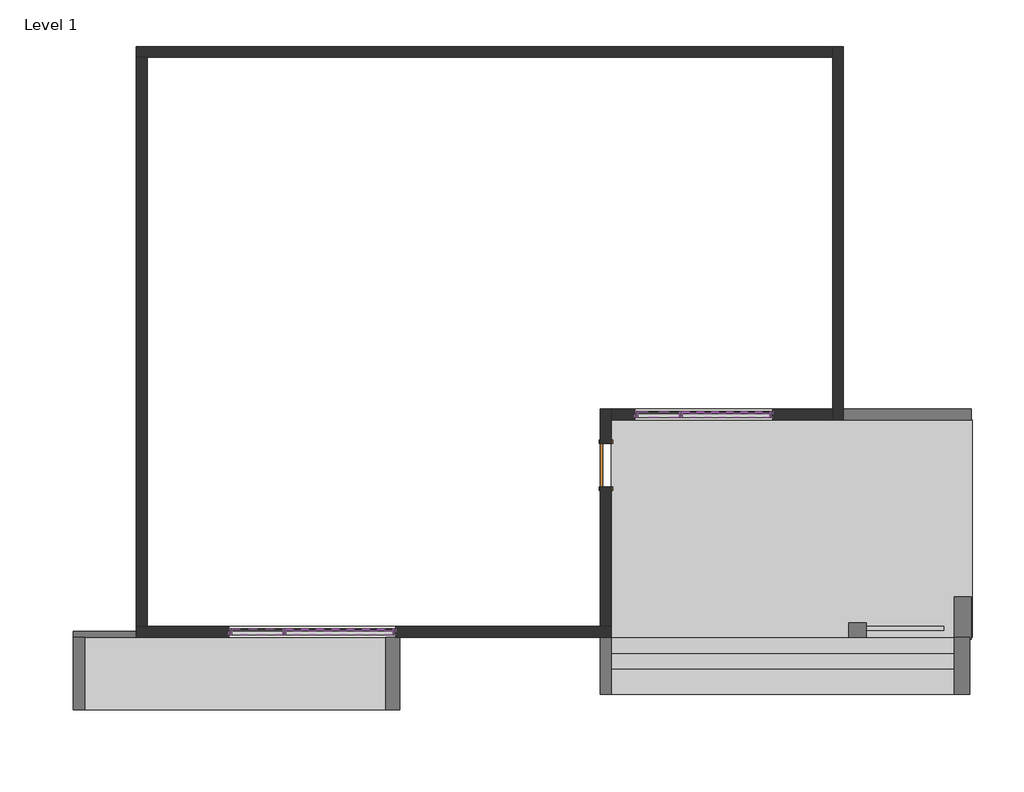
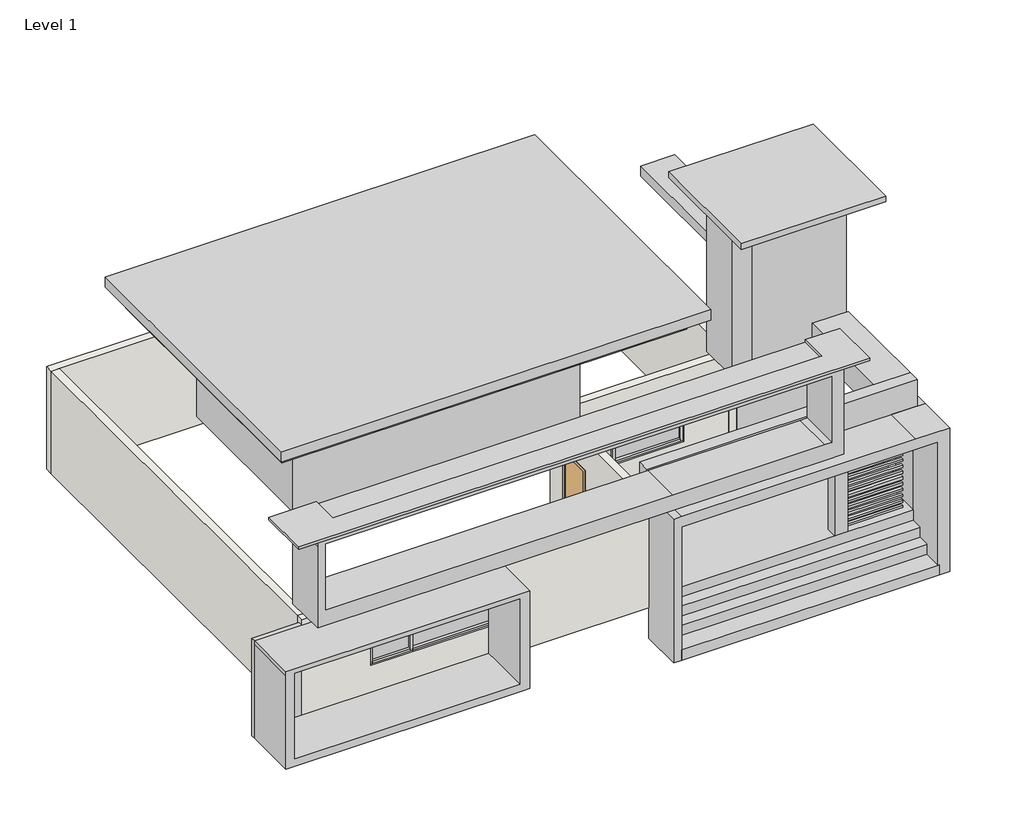
# One storey: 30 members, 8 plates, 6 walls, 5 proxies, 1 door.
"""IFC4 building model written with IfcOpenShell, lengths in millimetres."""

from ifc_helpers import new_model, si_unit, frame, origin, origin_with_axes, place, context, project, spatial, polyline, outline, extrude, faceted_brep, transform, mapped, element, save
from components import generic_models_1_generic_models_1_d0396bf3, generic_models_2_generic_models_2_1e60c849, generic_models_4_generic_models_4_de5db2ce, generic_models_5_generic_models_5_34eadfb7, generic_models_6_generic_models_6_aa42e9c5, door_0ca8825f, member_94e27682, member_024c663a, member_255fa45d, member_75351bdb, member_163b98ee, member_61d667c8, member_4d6ef9b1, member_f3803a17, member_1b8782c9, member_88cd697c, system_panel_glazed_c3c389f2, system_panel_glazed_f495917c, system_panel_glazed_3dd2ea40, system_panel_glazed_ce1b7c8d, system_panel_glazed_f70c9889, system_panel_glazed_55be9c8f

model = new_model("IFC4")

# Units and contexts
model_context = context("Model", 3, world=origin())
ifc_project = project(units=[si_unit("LENGTHUNIT", "METRE", prefix="MILLI")], contexts=[model_context])

# Site, building, storey
site = spatial("IfcSite", under=ifc_project)
building = spatial("IfcBuilding", under=site)
storey = spatial("IfcBuildingStorey", under=building, Name="Level 1", Elevation=0.0)

# Proxies
placement = place(None, origin())
generic_models_1_generic_models_1_shape = generic_models_1_generic_models_1_d0396bf3(model_context)
element("IfcBuildingElementProxy", 1, Name="Generic Models 1 : Generic Models 1", ObjectType="Generic Models 1 : Generic Models 1", at=placement, inside=storey, context=model_context, shape_type="MappedRepresentation", body=[
    mapped(generic_models_1_generic_models_1_shape, transform((0.0, 0.0, 0.0), x_axis=(1.0, 0.0, 0.0), y_axis=(0.0, 1.0, 0.0), z_axis=(0.0, 0.0, 1.0))),
])
generic_models_2_generic_models_2_shape = generic_models_2_generic_models_2_1e60c849(model_context)
element("IfcBuildingElementProxy", 2, Name="Generic Models 2 : Generic Models 2", ObjectType="Generic Models 2 : Generic Models 2", at=placement, inside=storey, context=model_context, shape_type="MappedRepresentation", body=[
    mapped(generic_models_2_generic_models_2_shape, transform((0.0, 0.0, 0.0), x_axis=(1.0, 0.0, 0.0), y_axis=(0.0, 1.0, 0.0), z_axis=(0.0, 0.0, 1.0))),
])
generic_models_4_generic_models_4_shape = generic_models_4_generic_models_4_de5db2ce(model_context)
element("IfcBuildingElementProxy", 3, Name="Generic Models 4 : Generic Models 4", ObjectType="Generic Models 4 : Generic Models 4", at=placement, inside=storey, context=model_context, shape_type="MappedRepresentation", body=[
    mapped(generic_models_4_generic_models_4_shape, transform((0.0, 0.0, 0.0), x_axis=(1.0, 0.0, 0.0), y_axis=(0.0, 1.0, 0.0), z_axis=(0.0, 0.0, 1.0))),
])
generic_models_5_generic_models_5_shape = generic_models_5_generic_models_5_34eadfb7(model_context)
element("IfcBuildingElementProxy", 4, Name="Generic Models 5 : Generic Models 5", ObjectType="Generic Models 5 : Generic Models 5", at=placement, inside=storey, context=model_context, shape_type="MappedRepresentation", body=[
    mapped(generic_models_5_generic_models_5_shape, transform((0.0, 0.0, 0.0), x_axis=(1.0, 0.0, 0.0), y_axis=(0.0, 1.0, 0.0), z_axis=(0.0, 0.0, 1.0))),
])
generic_models_6_generic_models_6_shape = generic_models_6_generic_models_6_aa42e9c5(model_context)
element("IfcBuildingElementProxy", 5, Name="Generic Models 6 : Generic Models 6", ObjectType="Generic Models 6 : Generic Models 6", at=placement, inside=storey, context=model_context, shape_type="MappedRepresentation", body=[
    mapped(generic_models_6_generic_models_6_shape, transform((0.0, 0.0, 0.0), x_axis=(1.0, 0.0, 0.0), y_axis=(0.0, 1.0, 0.0), z_axis=(0.0, 0.0, 1.0))),
])

# Door
door_shape = door_0ca8825f(model_context)
element("IfcDoor", 6, ObjectType="Single-Flush : 36\" x 84\"", at=placement, inside=storey, context=model_context, shape_type="MappedRepresentation", body=[
    mapped(door_shape, transform((-7974.5229687, -7170.2015118, 0.0), x_axis=(0.0, 1.0, 0.0), y_axis=(-1.0, 0.0, 0.0), z_axis=(0.0, 0.0, 1.0))),
])

# Members
member_shape = member_94e27682(model_context)
element("IfcMember", 7, ObjectType="Rectangular Mullion : 2.5\" x 5\" rectangular", at=placement, inside=storey, context=model_context, shape_type="MappedRepresentation", body=[
    mapped(member_shape, transform((-7364.9229687, -6103.4015118, 1983.9447059), x_axis=(-1.0, 0.0, 0.0), y_axis=(0.0, -1.0, 0.0), z_axis=(0.0, 0.0, 1.0))),
])
element("IfcMember", 8, ObjectType="Rectangular Mullion : 2.5\" x 5\" rectangular", at=placement, inside=storey, context=model_context, shape_type="MappedRepresentation", body=[
    mapped(member_shape, transform((-7364.9229687, -6103.4015118, 1439.8060341), x_axis=(-1.0, 0.0, 0.0), y_axis=(0.0, -1.0, 0.0), z_axis=(0.0, 0.0, 1.0))),
])
member_2_shape = member_024c663a(model_context)
element("IfcMember", 9, ObjectType="Rectangular Mullion : 2.5\" x 5\" rectangular", at=placement, inside=storey, context=model_context, shape_type="MappedRepresentation", body=[
    mapped(member_2_shape, transform((-7301.4229687, -6103.4015118, 895.6673623), x_axis=(0.0, 0.0, -1.0), y_axis=(0.0, -1.0, 0.0), z_axis=(-1.0, 0.0, 0.0))),
])
member_3_shape = member_255fa45d(model_context)
element("IfcMember", 10, ObjectType="Rectangular Mullion : 2.5\" x 5\" rectangular", at=placement, inside=storey, context=model_context, shape_type="MappedRepresentation", body=[
    mapped(member_3_shape, transform((-6399.7229687, -6103.4015118, 1439.8060341), x_axis=(1.0, 0.0, 0.0), y_axis=(0.0, -1.0, 0.0), z_axis=(0.0, 0.0, -1.0))),
])
element("IfcMember", 11, ObjectType="Rectangular Mullion : 2.5\" x 5\" rectangular", at=placement, inside=storey, context=model_context, shape_type="MappedRepresentation", body=[
    mapped(member_3_shape, transform((-6399.7229687, -6103.4015118, 895.6673623), x_axis=(1.0, 0.0, 0.0), y_axis=(0.0, -1.0, 0.0), z_axis=(0.0, 0.0, -1.0))),
])
element("IfcMember", 12, ObjectType="Rectangular Mullion : 2.5\" x 5\" rectangular", at=placement, inside=storey, context=model_context, shape_type="MappedRepresentation", body=[
    mapped(member_3_shape, transform((-6399.7229687, -6103.4015118, 1983.9447059), x_axis=(1.0, 0.0, 0.0), y_axis=(0.0, -1.0, 0.0), z_axis=(0.0, 0.0, -1.0))),
])
element("IfcMember", 13, ObjectType="Rectangular Mullion : 2.5\" x 5\" rectangular", at=placement, inside=storey, context=model_context, shape_type="MappedRepresentation", body=[
    mapped(member_2_shape, transform((-6431.4729687, -6103.4015118, 2528.0833777), x_axis=(0.0, 0.0, 1.0), y_axis=(0.0, -1.0, 0.0), z_axis=(1.0, 0.0, 0.0))),
])
element("IfcMember", 14, ObjectType="Rectangular Mullion : 2.5\" x 5\" rectangular", at=placement, inside=storey, context=model_context, shape_type="MappedRepresentation", body=[
    mapped(member_shape, transform((-7364.9229687, -6103.4015118, 2528.0833777), x_axis=(-1.0, 0.0, 0.0), y_axis=(0.0, -1.0, 0.0), z_axis=(0.0, 0.0, 1.0))),
])
member_4_shape = member_75351bdb(model_context)
element("IfcMember", 15, ObjectType="Rectangular Mullion : 2.5\" x 5\" rectangular", at=placement, inside=storey, context=model_context, shape_type="MappedRepresentation", body=[
    mapped(member_4_shape, transform((-6367.9729687, -6103.4015118, 895.6673623), x_axis=(0.0, 0.0, -1.0), y_axis=(0.0, -1.0, 0.0), z_axis=(-1.0, 0.0, 0.0))),
])
member_5_shape = member_163b98ee(model_context)
element("IfcMember", 16, ObjectType="Rectangular Mullion : 2.5\" x 5\" rectangular", at=placement, inside=storey, context=model_context, shape_type="MappedRepresentation", body=[
    mapped(member_5_shape, transform((-4532.8229687, -6103.4015118, 1983.9447059), x_axis=(0.0, 0.0, 1.0), y_axis=(0.0, -1.0, 0.0), z_axis=(1.0, 0.0, 0.0))),
])
element("IfcMember", 17, ObjectType="Rectangular Mullion : 2.5\" x 5\" rectangular", at=placement, inside=storey, context=model_context, shape_type="MappedRepresentation", body=[
    mapped(member_5_shape, transform((-4532.8229687, -6103.4015118, 1439.8060341), x_axis=(0.0, 0.0, 1.0), y_axis=(0.0, -1.0, 0.0), z_axis=(1.0, 0.0, 0.0))),
])
element("IfcMember", 18, ObjectType="Rectangular Mullion : 2.5\" x 5\" rectangular", at=placement, inside=storey, context=model_context, shape_type="MappedRepresentation", body=[
    mapped(member_4_shape, transform((-4532.8229687, -6103.4015118, 2528.0833777), x_axis=(0.0, 0.0, 1.0), y_axis=(0.0, -1.0, 0.0), z_axis=(1.0, 0.0, 0.0))),
])
element("IfcMember", 19, ObjectType="Rectangular Mullion : 2.5\" x 5\" rectangular", at=placement, inside=storey, context=model_context, shape_type="MappedRepresentation", body=[
    mapped(member_shape, transform((-4469.3229687, -6103.4015118, 1439.8060341), x_axis=(1.0, 0.0, 0.0), y_axis=(0.0, -1.0, 0.0), z_axis=(0.0, 0.0, -1.0))),
])
element("IfcMember", 20, ObjectType="Rectangular Mullion : 2.5\" x 5\" rectangular", at=placement, inside=storey, context=model_context, shape_type="MappedRepresentation", body=[
    mapped(member_shape, transform((-4469.3229687, -6103.4015118, 1983.9447059), x_axis=(1.0, 0.0, 0.0), y_axis=(0.0, -1.0, 0.0), z_axis=(0.0, 0.0, -1.0))),
])
element("IfcMember", 21, ObjectType="Rectangular Mullion : 2.5\" x 5\" rectangular", at=placement, inside=storey, context=model_context, shape_type="MappedRepresentation", body=[
    mapped(member_shape, transform((-4469.3229687, -6103.4015118, 895.6673623), x_axis=(1.0, 0.0, 0.0), y_axis=(0.0, -1.0, 0.0), z_axis=(0.0, 0.0, -1.0))),
])
member_6_shape = member_61d667c8(model_context)
element("IfcMember", 22, ObjectType="Rectangular Mullion : 2.5\" x 5\" rectangular", at=placement, inside=storey, context=model_context, shape_type="MappedRepresentation", body=[
    mapped(member_6_shape, transform((-15899.3229687, -10675.4015118, 2116.0432119), x_axis=(-1.0, 0.0, 0.0), y_axis=(0.0, -1.0, 0.0), z_axis=(0.0, 0.0, 1.0))),
])
element("IfcMember", 23, ObjectType="Rectangular Mullion : 2.5\" x 5\" rectangular", at=placement, inside=storey, context=model_context, shape_type="MappedRepresentation", body=[
    mapped(member_6_shape, transform((-15899.3229687, -10675.4015118, 1567.0065378), x_axis=(-1.0, 0.0, 0.0), y_axis=(0.0, -1.0, 0.0), z_axis=(0.0, 0.0, 1.0))),
])
member_7_shape = member_4d6ef9b1(model_context)
element("IfcMember", 24, ObjectType="Rectangular Mullion : 2.5\" x 5\" rectangular", at=placement, inside=storey, context=model_context, shape_type="MappedRepresentation", body=[
    mapped(member_7_shape, transform((-15835.8229687, -10675.4015118, 1017.9698638), x_axis=(0.0, 0.0, -1.0), y_axis=(0.0, -1.0, 0.0), z_axis=(-1.0, 0.0, 0.0))),
])
member_8_shape = member_f3803a17(model_context)
element("IfcMember", 25, ObjectType="Rectangular Mullion : 2.5\" x 5\" rectangular", at=placement, inside=storey, context=model_context, shape_type="MappedRepresentation", body=[
    mapped(member_8_shape, transform((-14730.9229687, -10675.4015118, 1017.9698638), x_axis=(1.0, 0.0, 0.0), y_axis=(0.0, -1.0, 0.0), z_axis=(0.0, 0.0, -1.0))),
])
element("IfcMember", 26, ObjectType="Rectangular Mullion : 2.5\" x 5\" rectangular", at=placement, inside=storey, context=model_context, shape_type="MappedRepresentation", body=[
    mapped(member_8_shape, transform((-14730.9229687, -10675.4015118, 1567.0065378), x_axis=(1.0, 0.0, 0.0), y_axis=(0.0, -1.0, 0.0), z_axis=(0.0, 0.0, -1.0))),
])
element("IfcMember", 27, ObjectType="Rectangular Mullion : 2.5\" x 5\" rectangular", at=placement, inside=storey, context=model_context, shape_type="MappedRepresentation", body=[
    mapped(member_8_shape, transform((-14730.9229687, -10675.4015118, 2116.0432119), x_axis=(1.0, 0.0, 0.0), y_axis=(0.0, -1.0, 0.0), z_axis=(0.0, 0.0, -1.0))),
])
element("IfcMember", 28, ObjectType="Rectangular Mullion : 2.5\" x 5\" rectangular", at=placement, inside=storey, context=model_context, shape_type="MappedRepresentation", body=[
    mapped(member_7_shape, transform((-14762.6729687, -10675.4015118, 2665.0798859), x_axis=(0.0, 0.0, 1.0), y_axis=(0.0, -1.0, 0.0), z_axis=(1.0, 0.0, 0.0))),
])
element("IfcMember", 29, ObjectType="Rectangular Mullion : 2.5\" x 5\" rectangular", at=placement, inside=storey, context=model_context, shape_type="MappedRepresentation", body=[
    mapped(member_6_shape, transform((-15899.3229687, -10675.4015118, 2665.0798859), x_axis=(-1.0, 0.0, 0.0), y_axis=(0.0, -1.0, 0.0), z_axis=(0.0, 0.0, 1.0))),
])
member_9_shape = member_1b8782c9(model_context)
element("IfcMember", 30, ObjectType="Rectangular Mullion : 2.5\" x 5\" rectangular", at=placement, inside=storey, context=model_context, shape_type="MappedRepresentation", body=[
    mapped(member_9_shape, transform((-14699.1729687, -10675.4015118, 1017.9698638), x_axis=(0.0, 0.0, -1.0), y_axis=(0.0, -1.0, 0.0), z_axis=(-1.0, 0.0, 0.0))),
])
member_10_shape = member_88cd697c(model_context)
element("IfcMember", 31, ObjectType="Rectangular Mullion : 2.5\" x 5\" rectangular", at=placement, inside=storey, context=model_context, shape_type="MappedRepresentation", body=[
    mapped(member_10_shape, transform((-12457.6229687, -10675.4015118, 1567.0065378), x_axis=(0.0, 0.0, 1.0), y_axis=(0.0, -1.0, 0.0), z_axis=(1.0, 0.0, 0.0))),
])
element("IfcMember", 32, ObjectType="Rectangular Mullion : 2.5\" x 5\" rectangular", at=placement, inside=storey, context=model_context, shape_type="MappedRepresentation", body=[
    mapped(member_10_shape, transform((-12457.6229687, -10675.4015118, 2116.0432119), x_axis=(0.0, 0.0, 1.0), y_axis=(0.0, -1.0, 0.0), z_axis=(1.0, 0.0, 0.0))),
])
element("IfcMember", 33, ObjectType="Rectangular Mullion : 2.5\" x 5\" rectangular", at=placement, inside=storey, context=model_context, shape_type="MappedRepresentation", body=[
    mapped(member_9_shape, transform((-12457.6229687, -10675.4015118, 2665.0798859), x_axis=(0.0, 0.0, 1.0), y_axis=(0.0, -1.0, 0.0), z_axis=(1.0, 0.0, 0.0))),
])
element("IfcMember", 34, ObjectType="Rectangular Mullion : 2.5\" x 5\" rectangular", at=placement, inside=storey, context=model_context, shape_type="MappedRepresentation", body=[
    mapped(member_6_shape, transform((-12394.1229687, -10675.4015118, 1567.0065378), x_axis=(1.0, 0.0, 0.0), y_axis=(0.0, -1.0, 0.0), z_axis=(0.0, 0.0, -1.0))),
])
element("IfcMember", 35, ObjectType="Rectangular Mullion : 2.5\" x 5\" rectangular", at=placement, inside=storey, context=model_context, shape_type="MappedRepresentation", body=[
    mapped(member_6_shape, transform((-12394.1229687, -10675.4015118, 2116.0432119), x_axis=(1.0, 0.0, 0.0), y_axis=(0.0, -1.0, 0.0), z_axis=(0.0, 0.0, -1.0))),
])
element("IfcMember", 36, ObjectType="Rectangular Mullion : 2.5\" x 5\" rectangular", at=placement, inside=storey, context=model_context, shape_type="MappedRepresentation", body=[
    mapped(member_6_shape, transform((-12394.1229687, -10675.4015118, 1017.9698638), x_axis=(1.0, 0.0, 0.0), y_axis=(0.0, -1.0, 0.0), z_axis=(0.0, 0.0, -1.0))),
])

# Plates
system_panel_glazed_shape = system_panel_glazed_c3c389f2(model_context)
element("IfcPlate", 37, ObjectType="System Panel : Glazed", at=placement, inside=storey, context=model_context, shape_type="MappedRepresentation", body=[
    mapped(system_panel_glazed_shape, transform((-6866.4479687, -6103.4015118, 959.1673623), x_axis=(1.0, 0.0, 0.0), y_axis=(0.0, 1.0, 0.0), z_axis=(0.0, 0.0, 1.0))),
])
system_panel_glazed_2_shape = system_panel_glazed_f495917c(model_context)
element("IfcPlate", 38, ObjectType="System Panel : Glazed", at=placement, inside=storey, context=model_context, shape_type="MappedRepresentation", body=[
    mapped(system_panel_glazed_2_shape, transform((-5450.3979687, -6103.4015118, 959.1673623), x_axis=(1.0, 0.0, 0.0), y_axis=(0.0, 1.0, 0.0), z_axis=(0.0, 0.0, 1.0))),
])
element("IfcPlate", 39, ObjectType="System Panel : Glazed", at=placement, inside=storey, context=model_context, shape_type="MappedRepresentation", body=[
    mapped(system_panel_glazed_2_shape, transform((-5450.3979687, -6103.4015118, 2015.6947059), x_axis=(1.0, 0.0, 0.0), y_axis=(0.0, 1.0, 0.0), z_axis=(0.0, 0.0, 1.0))),
])
system_panel_glazed_3_shape = system_panel_glazed_3dd2ea40(model_context)
element("IfcPlate", 40, ObjectType="System Panel : Glazed", at=placement, inside=storey, context=model_context, shape_type="MappedRepresentation", body=[
    mapped(system_panel_glazed_3_shape, transform((-5450.3979687, -6103.4015118, 1471.5560341), x_axis=(1.0, 0.0, 0.0), y_axis=(0.0, 1.0, 0.0), z_axis=(0.0, 0.0, 1.0))),
])
system_panel_glazed_4_shape = system_panel_glazed_ce1b7c8d(model_context)
element("IfcPlate", 41, ObjectType="System Panel : Glazed", at=placement, inside=storey, context=model_context, shape_type="MappedRepresentation", body=[
    mapped(system_panel_glazed_4_shape, transform((-15299.2479687, -10675.4015118, 1081.4698638), x_axis=(1.0, 0.0, 0.0), y_axis=(0.0, 1.0, 0.0), z_axis=(0.0, 0.0, 1.0))),
])
system_panel_glazed_5_shape = system_panel_glazed_f70c9889(model_context)
element("IfcPlate", 42, ObjectType="System Panel : Glazed", at=placement, inside=storey, context=model_context, shape_type="MappedRepresentation", body=[
    mapped(system_panel_glazed_5_shape, transform((-13578.3979687, -10675.4015118, 1081.4698638), x_axis=(1.0, 0.0, 0.0), y_axis=(0.0, 1.0, 0.0), z_axis=(0.0, 0.0, 1.0))),
])
element("IfcPlate", 43, ObjectType="System Panel : Glazed", at=placement, inside=storey, context=model_context, shape_type="MappedRepresentation", body=[
    mapped(system_panel_glazed_5_shape, transform((-13578.3979687, -10675.4015118, 2147.7932119), x_axis=(1.0, 0.0, 0.0), y_axis=(0.0, 1.0, 0.0), z_axis=(0.0, 0.0, 1.0))),
])
system_panel_glazed_6_shape = system_panel_glazed_55be9c8f(model_context)
element("IfcPlate", 44, ObjectType="System Panel : Glazed", at=placement, inside=storey, context=model_context, shape_type="MappedRepresentation", body=[
    mapped(system_panel_glazed_6_shape, transform((-13578.3979687, -10675.4015118, 1598.7565378), x_axis=(1.0, 0.0, 0.0), y_axis=(0.0, 1.0, 0.0), z_axis=(0.0, 0.0, 1.0))),
])

# Walls
element("IfcWall", 45, ObjectType="9\"", at=placement, inside=storey, context=model_context, shape_type="Brep", body=[
    faceted_brep([(-17842.4229687, -10789.7015118, 0.0), (-7860.2229687, -10789.7015118, 0.0), (-7860.2229687, -10789.7015118, 3048.0), (-17842.4229687, -10789.7015118, 3048.0), (-15899.3229687, -10789.7015118, 1017.9698638), (-15899.3229687, -10789.7015118, 2665.0798859), (-12394.1229687, -10789.7015118, 2665.0798859), (-12394.1229687, -10789.7015118, 1017.9698638), (-7860.2229687, -10561.1015118, 0.0), (-8088.8229687, -10561.1015118, 0.0), (-17613.8229687, -10561.1015118, 0.0), (-17842.4229687, -10561.1015118, 0.0), (-17842.4229687, -10561.1015118, 3048.0), (-17613.8229687, -10561.1015118, 3048.0), (-8088.8229687, -10561.1015118, 3048.0), (-7860.2229687, -10561.1015118, 3048.0), (-15899.3229687, -10561.1015118, 2665.0798859), (-15899.3229687, -10561.1015118, 1017.9698638), (-12394.1229687, -10561.1015118, 1017.9698638), (-12394.1229687, -10561.1015118, 2665.0798859)], [[[0, 1, 2, 3], [4, 5, 6, 7]], [[8, 9, 10, 11, 12, 13, 14, 15], [16, 17, 18, 19]], [[1, 0, 11, 10, 9, 8]], [[2, 1, 8, 15]], [[3, 2, 15, 14, 13, 12]], [[0, 3, 12, 11]], [[4, 17, 16, 5]], [[5, 16, 19, 6]], [[6, 19, 18, 7]], [[17, 4, 7, 18]]]),
])
element("IfcWall", 46, ObjectType="9\"", at=placement, inside=storey, context=model_context, shape_type="Brep", body=[
    faceted_brep([(-3212.0229687, 1630.8984882, 0.0), (-17842.4229687, 1630.8984882, 0.0), (-17842.4229687, 1630.8984882, 3048.0), (-3212.0229687, 1630.8984882, 3048.0), (-3212.0229687, 1402.2984882, 0.0), (-3212.0229687, 1402.2984882, 3048.0), (-17613.8229687, 1402.2984882, 3048.0), (-17842.4229687, 1402.2984882, 3048.0), (-17842.4229687, 1402.2984882, 0.0), (-17613.8229687, 1402.2984882, 0.0)], [[[0, 1, 2, 3]], [[4, 5, 6, 7, 8, 9]], [[1, 0, 4, 9, 8]], [[3, 2, 7, 6, 5]], [[0, 3, 5, 4]], [[2, 1, 8, 7]]]),
])
element("IfcWall", 47, ObjectType="9\"", at=placement, inside=storey, context=model_context, shape_type="SweptSolid", body=[
    extrude(outline(polyline([(-17842.4229687, -10561.1015118), (-17842.4229687, 1402.2984882), (-17613.8229687, 1402.2984882), (-17613.8229687, -10561.1015118), (-17842.4229687, -10561.1015118)])), origin_with_axes(), (0.0, 0.0, 1.0), 3048.0),
])
element("IfcWall", 48, ObjectType="9\"", at=placement, inside=storey, context=model_context, shape_type="Brep", body=[
    faceted_brep([(-7860.2229687, -6713.0015118, 2133.6), (-7860.2229687, -6713.0015118, 0.0), (-7860.2229687, -6217.7015118, 0.0), (-7860.2229687, -5989.1015118, 0.0), (-7860.2229687, -5989.1015118, 3048.0), (-7860.2229687, -6217.7015118, 3048.0), (-7860.2229687, -10561.1015118, 3048.0), (-7860.2229687, -10561.1015118, 0.0), (-7860.2229687, -7627.4015118, 0.0), (-7860.2229687, -7627.4015118, 2133.6), (-8088.8229687, -5989.1015118, 0.0), (-8088.8229687, -6713.0015118, 0.0), (-8088.8229687, -6713.0015118, 2133.6), (-8088.8229687, -7627.4015118, 2133.6), (-8088.8229687, -7627.4015118, 0.0), (-8088.8229687, -10561.1015118, 0.0), (-8088.8229687, -10561.1015118, 3048.0), (-8088.8229687, -5989.1015118, 3048.0)], [[[0, 1, 2, 3, 4, 5, 6, 7, 8, 9]], [[10, 11, 12, 13, 14, 15, 16, 17]], [[8, 7, 15, 14]], [[3, 2, 1, 11, 10]], [[6, 5, 4, 17, 16]], [[7, 6, 16, 15]], [[4, 3, 10, 17]], [[12, 11, 1, 0]], [[13, 12, 0, 9]], [[14, 13, 9, 8]]]),
])
element("IfcWall", 49, ObjectType="9\"", at=placement, inside=storey, context=model_context, shape_type="SweptSolid", body=[
    extrude(outline(polyline([(0.0, -7860.2229687), (0.0, -3212.0229687), (3048.0, -3212.0229687), (3048.0, -7860.2229687), (0.0, -7860.2229687)]), holes=[polyline([(895.6673623, -7364.9229687), (2528.0833777, -7364.9229687), (2528.0833777, -4469.3229687), (895.6673623, -4469.3229687), (895.6673623, -7364.9229687)])]), frame((0.0, -6217.7015118, 0.0), z_axis=(0.0, 1.0, 0.0), x_axis=(0.0, 0.0, 1.0)), (0.0, 0.0, 1.0), 228.6),
])
element("IfcWall", 50, ObjectType="9\"", at=placement, inside=storey, context=model_context, shape_type="Brep", body=[
    faceted_brep([(-2983.4229687, -6217.7015118, 0.0), (-2983.4229687, 1630.8984882, 0.0), (-2983.4229687, 1630.8984882, 3048.0), (-2983.4229687, -6217.7015118, 3048.0), (-3212.0229687, -6217.7015118, 0.0), (-3212.0229687, -6217.7015118, 3048.0), (-3212.0229687, -5989.1015118, 3048.0), (-3212.0229687, 1402.2984882, 3048.0), (-3212.0229687, 1630.8984882, 3048.0), (-3212.0229687, 1630.8984882, 0.0), (-3212.0229687, 1402.2984882, 0.0), (-3212.0229687, -5989.1015118, 0.0)], [[[0, 1, 2, 3]], [[4, 5, 6, 7, 8, 9, 10, 11]], [[1, 0, 4, 11, 10, 9]], [[3, 2, 8, 7, 6, 5]], [[0, 3, 5, 4]], [[2, 1, 9, 8]]]),
])

save(model, "model.ifc")

# Revit data of these elements
# Type "Single-Flush : 36\" x 84\""
#   Type Mark = "1"
#   Construction Type Id = "MDOOR"
#   Assembly Code = "C1020"
#   Analytic Construction = "Metal"
#   Thickness = 0' - 2"
#   Heat Transfer Coefficient (U) = 0.651978 BTU/(h·ft²·°F)
#   Height = 7' - 0"
#   Trim Projection Ext = 0' - 1"
#   Trim Projection Int = 0' - 1"
#   Trim Width = 0' - 3"
#   Width = 3' - 0"
#   Define Thermal Properties by = 1
#   Define Thermal Properties by = 1
#   Door Material = Door - Panel
#   Frame Material = Door - Frame
#   Visual Light Transmittance = 0
#   Solar Heat Gain Coefficient = 0
#   Function = (empty or 0)
#   Wall Closure = (empty or 0)
# Type "Rectangular Mullion : 2.5\" x 5\" rectangular"
#   built-in parameter 1007304 = 0.416667 (stored number, unit not read)
#   built-in parameter 1007301 = 0.104167 (stored number, unit not read)
#   built-in parameter 1007300 = 0.104167 (stored number, unit not read)
# Type "System Panel : Glazed"
#   Construction Type Id = "GSP4R"
#   Analytic Construction = "1/8 in Pilkington single glazing"
#   Visual Light Transmittance = 0.9
#   Solar Heat Gain Coefficient = 0.86
#   Heat Transfer Coefficient (U) = 1.18115 BTU/(h·ft²·°F)
#   Define Thermal Properties by = 1
# Type "9\""
#   Assembly Code = "B2010"
#   Layers, outside or top first: 0' - 9" no material (function 1)
# Element 1 (IfcBuildingElementProxy, "Generic Models 1 : Generic Models 1")
#   Phase Created = New Construction
# Element 2 (IfcBuildingElementProxy, "Generic Models 2 : Generic Models 2")
#   Phase Created = New Construction
# Element 3 (IfcBuildingElementProxy, "Generic Models 4 : Generic Models 4")
#   Phase Created = New Construction
# Element 4 (IfcBuildingElementProxy, "Generic Models 5 : Generic Models 5")
#   Phase Created = New Construction
#   Materials on its faces: "Tile, Mosaic, Gray", "Tile, Porcelain, 4in"
# Element 5 (IfcBuildingElementProxy, "Generic Models 6 : Generic Models 6")
#   Phase Created = New Construction
# Element 6 (IfcDoor, "Single-Flush : 36\" x 84\"")
#   Phase Created = New Construction
#   Materials on its faces: "Door - Frame", "Door - Panel"
# Elements 7, 8, 9, 10, 11, 12, 13, 14, 15, 16, 17, 18, 19, 20, 21, 22, 23, 24, 25, 26, 27, 28, 29, 30, 31, 32, 33, 34, 35, 36 (IfcMember, "Rectangular Mullion : 2.5\" x 5\" rectangular")
#   Phase Created = New Construction
#   Materials on its faces: "Aluminum"
# Elements 37, 38, 39, 40, 41, 42, 43, 44 (IfcPlate, "System Panel : Glazed")
#   Phase Created = New Construction
#   Materials on its faces: "Glass"
# Elements 45, 46, 47, 48, 49, 50 (IfcWall, "9\"")
#   Top Offset = 0' - 0"
#   Base Offset = 0' - 0"
#   Unconnected Height = 10' - 0"
#   wall height = 10' - 0"
#   Phase Created = New Construction
#   Base Constraint = Level 1
#   Materials on its faces: "Default Wall"
# Materials
#   "Door - Panel": class "Wood", colour RGB 210 159 95, transparency 0, Cost = 0
#   "Door - Frame": colour RGB 118 70 51, transparency 0, Cost = 0
#   "Tile, Mosaic, Gray": class "Generic", colour RGB 127 127 127, transparency 0, Description = "Mosiac tile, gray", Cost = 0
#   "Tile, Porcelain, 4in": class "Generic", colour RGB 89 87 158, transparency 0, Description = "Porcelain tile, 4\", white", Cost = 0
#   "Aluminum": class "Metal", colour RGB 247 247 247, transparency 0, Description = "Aluminum 6061", Cost = 0
#   "Glass": class "Glass", colour RGB 0 128 192, transparency 0.75, Description = "Soda Lime Glass", Cost = 0
#   "Default Wall": colour RGB 128 128 128, transparency 0, Cost = 0
